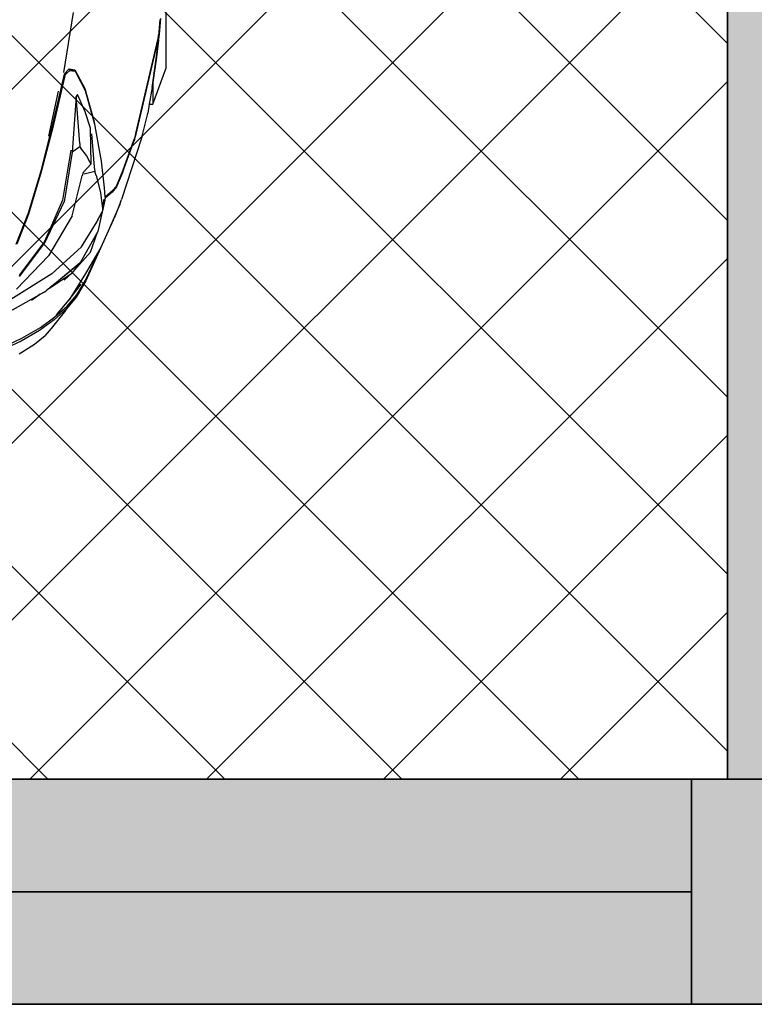
# Model space of a CAD drawing. Units: inches. Extents: x 2167 to 2589, y 1680 to 2489.
# Tile 14 of 38: x 2389 to 2419, y 1688 to 1727. Entities that reach past the tile are written whole.
import ezdxf

# ---------------------------------------------------------------- set-up
doc = ezdxf.new("R2010")
doc.units = ezdxf.units.IN
doc.header["$MEASUREMENT"] = 0
doc.layers.get('0').update_dxf_attribs({"color": 250})
doc.layers.add('A-FLOR-PATT', color=254, linetype='Continuous', lineweight=13, true_color=0xfeeab9)
for name, color, linetype, lineweight in [('A-WALL-PATT', 250, 'Continuous', 13), ('C-PRKG-VEHS', 8, 'Continuous', 13), ('C-PROP', 7, 'Continuous', 35), ('L-PVMT-PATT', 252, 'Continuous', 13), ('walls', 7, 'Continuous', 35)]:
    doc.layers.add(name, color=color, linetype=linetype, lineweight=lineweight)
doc.layers.add('Edges', color=250, linetype='Continuous')

# ---------------------------------------------------------------- blocks, each defined once
blk = doc.blocks.new('Nissan Qashqai pl')
at = {"layer": 'Edges'}
for p, q in [((10.9577, 12.8101), (11.1283, 12.8101)), ((11.1783, 12.7921), (11.1283, 12.8101)), ((11.0576, 12.8026), (11.0798, 12.8008)), ((11.0768, 12.8008), (11.059, 12.8023)), ((11.0811, 12.8004), (11.0768, 12.8008)), ((11.0798, 12.8008), (11.0872, 12.7999)), ((11.0827, 12.8001), (11.0811, 12.8004)), ((11.0827, 12.8001), (11.0813, 12.7998)), ((11.0836, 12.8002), (11.0827, 12.8001)), ((11.0856, 12.7994), (11.0827, 12.8001)), ((11.0872, 12.7999), (11.0836, 12.8002)), ((11.0836, 12.8002), (11.0882, 12.7992)), ((11.2196, 12.7681), (11.0856, 12.7994)), ((11.0883, 12.7998), (11.0872, 12.7999)), ((11.0882, 12.7992), (11.2222, 12.7676)), ((11.0883, 12.7998), (11.1123, 12.797)), ((11.1147, 12.7965), (11.0883, 12.7998)), ((11.1123, 12.797), (11.1475, 12.7921)), ((11.1547, 12.791), (11.1147, 12.7965)), ((11.1475, 12.7921), (11.1525, 12.7914)), ((11.1475, 12.7921), (11.1783, 12.7921)), ((11.1525, 12.7914), (11.1547, 12.791)), ((11.1547, 12.791), (11.1783, 12.787)), ((11.1783, 12.787), (11.1783, 12.7921)), ((11.1783, 12.787), (11.1906, 12.7849)), ((11.1906, 12.7849), (11.1909, 12.7849)), ((11.193, 12.7845), (11.1909, 12.7849)), ((11.2215, 12.7775), (11.193, 12.7845)), ((11.2247, 12.767), (11.2163, 12.7689)), ((11.22, 12.768), (11.2196, 12.7681)), ((11.2247, 12.767), (11.22, 12.768)), ((11.2247, 12.7764), (11.2215, 12.7775)), ((11.2222, 12.7676), (11.2271, 12.7664)), ((11.2247, 12.7764), (11.3124, 12.7479)), ((11.2253, 12.7668), (11.2247, 12.767)), ((11.2304, 12.7649), (11.2253, 12.7668)), ((11.2253, 12.7668), (11.2271, 12.7664)), ((11.2271, 12.7664), (11.2296, 12.7658)), ((11.2271, 12.7664), (11.2277, 12.7662)), ((11.2277, 12.7662), (11.2296, 12.7658)), ((11.2732, 12.7496), (11.2277, 12.7662)), ((11.2704, 12.7504), (11.2304, 12.7649)), ((11.2702, 12.7507), (11.2704, 12.7504)), ((11.2704, 12.7506), (11.2707, 12.7503)), ((11.2707, 12.7503), (11.2704, 12.7504)), ((11.2719, 12.7498), (11.2707, 12.7503)), ((11.2934, 12.741), (11.2719, 12.7498)), ((11.2732, 12.7496), (11.2946, 12.7409)), ((11.3, 12.735), (11.2934, 12.741)), ((11.2946, 12.7409), (11.3018, 12.7346)), ((11.3161, 12.7467), (11.3124, 12.7479)), ((11.3161, 12.7467), (11.3376, 12.7381)), ((11.3192, 12.7454), (11.3566, 12.7294)), ((11.3081, 12.7253), (11.3, 12.735)), ((11.3018, 12.7346), (11.3103, 12.7249)), ((11.3086, 12.7247), (11.3081, 12.7253)), ((11.3081, 12.7253), (11.3087, 12.7247)), ((11.3103, 12.7249), (11.3103, 12.7249)), ((11.3405, 12.7369), (11.3376, 12.7381)), ((11.3405, 12.7369), (11.3566, 12.7294)), ((11.3566, 12.7294), (11.3796, 12.7187)), ((11.2091, 12.7103), (11.2583, 12.7196)), ((11.2583, 12.7196), (11.2956, 12.7234)), ((11.2787, 12.7123), (11.2729, 12.7104)), ((11.2787, 12.7123), (11.3022, 12.7186)), ((11.2956, 12.7234), (11.3085, 12.7247)), ((11.3022, 12.7186), (11.3252, 12.7213)), ((11.3085, 12.7247), (11.3086, 12.7247)), ((11.3086, 12.7247), (11.3087, 12.7247)), ((11.3087, 12.7247), (11.3103, 12.7249)), ((11.3103, 12.7249), (11.3106, 12.7249)), ((11.3106, 12.7249), (11.314, 12.7238)), ((11.317, 12.7227), (11.3119, 12.7236)), ((11.3132, 12.7243), (11.3256, 12.7215)), ((11.314, 12.7238), (11.317, 12.7227)), ((11.314, 12.7238), (11.3242, 12.7216)), ((11.3242, 12.7216), (11.317, 12.7227)), ((11.3198, 12.7211), (11.3252, 12.7213)), ((11.3242, 12.7216), (11.3256, 12.7215)), ((11.3252, 12.7213), (11.3283, 12.7214)), ((11.3256, 12.7215), (11.3283, 12.7214)), ((11.3283, 12.7214), (11.3297, 12.7206)), ((11.3297, 12.7206), (11.3446, 12.7173)), ((11.3297, 12.7206), (11.3302, 12.7203)), ((11.3302, 12.7203), (11.3446, 12.7173)), ((11.3302, 12.7203), (11.3394, 12.7152)), ((11.3394, 12.7152), (11.3434, 12.7138)), ((11.3394, 12.7152), (11.342, 12.7137)), ((11.379, 12.6915), (11.3434, 12.7138)), ((11.3446, 12.7173), (11.3571, 12.7146)), ((11.3583, 12.7142), (11.3571, 12.7146)), ((11.3571, 12.7146), (11.3821, 12.7008)), ((11.3583, 12.7142), (11.3821, 12.7008)), ((11.3864, 12.7044), (11.3583, 12.7142)), ((11.3796, 12.7187), (11.4164, 12.6974)), ((11.3796, 12.7187), (11.3807, 12.7182)), ((11.3807, 12.7182), (11.4267, 12.6979)), ((11.4228, 12.6989), (11.3807, 12.7182)), ((11.156, 12.6966), (11.203, 12.7093)), ((11.1589, 12.6971), (11.2062, 12.7098)), ((11.2121, 12.7043), (11.189, 12.6968)), ((11.203, 12.7093), (11.2091, 12.7103)), ((11.2062, 12.7098), (11.2091, 12.7103)), ((11.2622, 12.7051), (11.2121, 12.7043)), ((11.2199, 12.706), (11.2666, 12.7097)), ((11.2505, 12.6987), (11.2401, 12.6908)), ((11.2601, 12.7037), (11.2505, 12.6987)), ((11.2622, 12.7051), (11.2601, 12.7037)), ((11.2743, 12.6942), (11.2622, 12.7051)), ((11.2666, 12.7097), (11.2729, 12.7104)), ((11.2729, 12.7104), (11.2766, 12.6957)), ((11.3821, 12.7008), (11.4014, 12.69)), ((11.4163, 12.6775), (11.3864, 12.7044)), ((11.4164, 12.6974), (11.4531, 12.6744)), ((11.4243, 12.6982), (11.4228, 12.6989)), ((11.4464, 12.6853), (11.4243, 12.6982)), ((11.4267, 12.6979), (11.4498, 12.6844)), ((11.1298, 12.6823), (11.156, 12.6966)), ((11.1319, 12.6827), (11.1365, 12.6851)), ((11.1365, 12.6851), (11.1589, 12.6971)), ((11.189, 12.6968), (11.1644, 12.6862)), ((11.1644, 12.6862), (11.1672, 12.6844)), ((11.2337, 12.6892), (11.1672, 12.6844)), ((11.1672, 12.6844), (11.2459, 12.6785)), ((11.2337, 12.6892), (11.2382, 12.6892)), ((11.2382, 12.6892), (11.2401, 12.6908)), ((11.2382, 12.6892), (11.2459, 12.6785)), ((11.2743, 12.6942), (11.2791, 12.6927)), ((11.335, 12.6786), (11.2791, 12.6927)), ((11.379, 12.6915), (11.417, 12.6499)), ((11.4014, 12.69), (11.4022, 12.6894)), ((11.4014, 12.69), (11.4265, 12.6594)), ((11.4022, 12.6894), (11.4163, 12.6775)), ((11.4022, 12.6894), (11.4265, 12.6594)), ((11.4531, 12.6744), (11.4314, 12.6911)), ((11.4624, 12.6717), (11.4464, 12.6853)), ((11.4498, 12.6844), (11.4662, 12.6706)), ((11.4681, 12.6691), (11.4498, 12.6844)), ((11.1336, 12.667), (11.0492, 12.6807)), ((11.1285, 12.6745), (11.1298, 12.6823)), ((11.1293, 12.6736), (11.1285, 12.6745)), ((11.1306, 12.6812), (11.1293, 12.6736)), ((11.1353, 12.6677), (11.1293, 12.6736)), ((11.1306, 12.6752), (11.1319, 12.6827)), ((11.1319, 12.6827), (11.1306, 12.6812)), ((11.1347, 12.671), (11.1306, 12.6752)), ((11.1366, 12.6691), (11.1347, 12.671)), ((11.2428, 12.6769), (11.3132, 12.6652)), ((11.2459, 12.6785), (11.3153, 12.6672)), ((11.335, 12.6786), (11.3915, 12.6453)), ((11.4366, 12.6471), (11.4163, 12.6775)), ((11.4163, 12.6775), (11.4259, 12.6674)), ((11.4742, 12.6567), (11.4531, 12.6744)), ((11.4774, 12.6543), (11.4624, 12.6717)), ((11.4662, 12.6706), (11.4815, 12.6531)), ((11.1358, 12.6676), (11.1353, 12.6677)), ((11.1358, 12.6676), (11.1366, 12.6691)), ((11.148, 12.665), (11.1358, 12.6676)), ((11.1401, 12.6682), (11.1366, 12.6691)), ((11.2066, 12.6527), (11.1401, 12.6682)), ((11.2063, 12.6515), (11.148, 12.665)), ((11.2232, 12.6458), (11.1598, 12.6594)), ((11.3132, 12.6652), (11.3715, 12.6398)), ((11.3733, 12.6404), (11.3153, 12.6672)), ((11.4265, 12.6594), (11.4366, 12.6471)), ((11.4681, 12.6691), (11.4936, 12.6491)), ((11.272, 12.6349), (11.2063, 12.6515)), ((11.2728, 12.6357), (11.2066, 12.6527)), ((11.3915, 12.6453), (11.4381, 12.6002)), ((11.417, 12.6499), (11.4529, 12.5922)), ((11.4366, 12.6471), (11.4408, 12.6419)), ((11.4408, 12.6419), (11.4411, 12.6414)), ((11.4924, 12.6339), (11.4774, 12.6543)), ((11.4815, 12.6531), (11.4963, 12.6328)), ((11.4936, 12.6491), (11.5033, 12.6408)), ((11.3311, 12.6172), (11.272, 12.6349)), ((11.3323, 12.6178), (11.2728, 12.6357)), ((11.3715, 12.6398), (11.4177, 12.6052)), ((11.4203, 12.6044), (11.3733, 12.6404)), ((11.4411, 12.6414), (11.4411, 12.6414)), ((11.4414, 12.6409), (11.4411, 12.6414)), ((11.4414, 12.6409), (11.447, 12.6315)), ((11.4455, 12.6336), (11.4414, 12.6409)), ((11.447, 12.6315), (11.4455, 12.6336)), ((11.4455, 12.6336), (11.4462, 12.6324)), ((11.447, 12.6315), (11.4462, 12.6324)), ((11.4732, 12.585), (11.4462, 12.6324)), ((11.447, 12.6315), (11.447, 12.6314)), ((11.4536, 12.6215), (11.447, 12.6314)), ((11.5074, 12.608), (11.4924, 12.6339)), ((11.4964, 12.6326), (11.4963, 12.6328)), ((11.4964, 12.6326), (11.5113, 12.6069)), ((11.5158, 12.6256), (11.5033, 12.6408)), ((11.3751, 12.5999), (11.3311, 12.6172)), ((11.3747, 12.6011), (11.3323, 12.6178)), ((11.5295, 12.6041), (11.5158, 12.6256)), ((11.4177, 12.6052), (11.4193, 12.6042)), ((11.5165, 12.5882), (11.5074, 12.608)), ((11.5113, 12.6068), (11.5113, 12.6069)), ((11.5113, 12.6068), (11.5206, 12.5869))]:
    blk.add_line(p, q, dxfattribs=at)
blk = doc.blocks.new('car')
blk.add_blockref('Nissan Qashqai pl', (-9.7433, -11.9151))
blk = doc.blocks.new('carr')
blk.add_blockref('car', (0.5124, -0.007))

msp = doc.modelspace()

# ---------------------------------------------------------------- hatches: boundary and pattern name
at = {"layer": 'A-FLOR-PATT'}
h = msp.add_hatch(color=256, dxfattribs=at)
h.dxf.hatch_style = 1
h.paths.add_polyline_path([(2525.548, 1864.695), (2455.041, 1864.695), (2455.041, 1855.153), (2455.041, 1830.653), (2525.548, 1830.653)])
h.paths.add_polyline_path([(2455.041, 1855.153), (2452.048, 1855.153), (2452.048, 1864.695), (2426.208, 1864.695), (2422.048, 1864.695), (2422.048, 1788.195), (2467.347, 1788.195), (2467.347, 1812.195), (2452.048, 1812.195), (2452.048, 1830.653), (2455.041, 1830.653)])
h.paths.add_polyline_path([(2419.685, 1779.195), (2417.548, 1779.195), (2417.548, 1696.695), (2419.685, 1696.695)])
at = {"layer": 'A-WALL-PATT'}
h = msp.add_hatch(color=256, dxfattribs=at)
h.dxf.hatch_style = 1
h.paths.add_polyline_path([(2575.048, 2029.695), (2422.048, 2029.695), (2422.048, 2161.695), (2427.018, 2161.695), (2427.018, 2161.941), (2427.018, 2166.195), (2417.548, 2166.195), (2417.548, 2025.195), (2575.048, 2025.195)])
h.paths.add_polyline_path([(2575.048, 2166.195), (2503.006, 2166.195), (2503.006, 2161.695), (2575.048, 2161.695)], flags=17)
h.paths.add_polyline_path([(2575.048, 2161.695), (2566.048, 2161.695), (2566.048, 2029.695), (2575.048, 2029.695)], flags=17)
h.paths.add_polyline_path([(2575.048, 2025.195), (2566.048, 2025.195), (2566.048, 1869.195), (2575.048, 1869.195)])
h.paths.add_polyline_path([(2575.048, 1869.195), (2566.048, 1869.195), (2447.7, 1869.195, -0.014764), (2447.737, 1867.924), (2447.737, 1864.695), (2575.048, 1864.695)])
h.paths.add_polyline_path([(2530.048, 1864.695), (2525.548, 1864.695), (2525.548, 1816.695), (2452.048, 1816.695), (2452.048, 1812.195), (2530.048, 1812.195)])
h.paths.add_polyline_path([(2455.041, 1830.653), (2452.048, 1830.653), (2452.048, 1816.695), (2455.041, 1816.695)], flags=17)
h.paths.add_polyline_path([(2575.048, 1864.695), (2566.048, 1864.695), (2566.048, 1788.195), (2456.097, 1788.195), (2456.097, 1783.941, -0.042065), (2455.697, 1779.195), (2527.685, 1779.195), (2527.685, 1687.695), (2532.185, 1687.695), (2532.185, 1779.195), (2575.048, 1779.195)])
h.paths.add_polyline_path([(2421.872, 1696.695), (2416.107, 1696.695), (2416.107, 1687.695), (2421.872, 1687.695)])
h.paths.add_polyline_path([(2375.607, 1696.695), (2369.843, 1696.695), (2369.843, 1687.695), (2375.607, 1687.695)])
h.paths.add_polyline_path([(2425.048, 2245.695), (2420.548, 2245.695), (2420.548, 2226.195), (2432.286, 2226.195), (2432.286, 2229.424), (2432.286, 2230.695), (2425.048, 2230.695)])
h.paths.add_polyline_path([(2224.048, 2151.195), (2318.548, 2151.195), (2318.548, 2177.304), (2314.783, 2177.304, -0.007324), (2314.048, 2177.315), (2314.048, 2155.695), (2224.048, 2155.695), (2224.048, 2157.455), (2215.048, 2157.455), (2215.048, 2103.585), (2218.974, 2103.585), (2224.048, 2103.585)])
at = {"layer": 'L-PVMT-PATT'}
h = msp.add_hatch(dxfattribs=at)
h.set_pattern_fill('ANSI37', color=256, scale=40)
h.paths.add_polyline_path([(2417.548, 1783.695), (2417.548, 1846.042), (2239.361, 1846.042), (2239.361, 1687.695), (2369.843, 1687.695), (2369.843, 1696.695), (2375.607, 1696.695), (2416.107, 1696.695), (2417.548, 1696.695)])
h = msp.add_hatch(color=256, dxfattribs=at)
h.dxf.hatch_style = 1
h.paths.add_polyline_path([(2416.107, 1696.695), (2375.607, 1696.695), (2375.607, 1692.195), (2416.107, 1692.195)])
h.paths.add_polyline_path([(2416.107, 1692.195), (2375.607, 1692.195), (2375.607, 1687.695), (2416.107, 1687.695)])

# ---------------------------------------------------------------- linework, layer by layer
at = {"layer": 'C-PROP'}
msp.add_line((2575.048, 1687.695), (2215.048, 1687.695), dxfattribs=at)
at = {"layer": 'walls'}
for p, q in [((2417.548, 1783.695), (2417.548, 1696.695)), ((2416.107, 1696.695), (2375.607, 1696.695)), ((2421.872, 1696.695), (2416.107, 1696.695)), ((2416.107, 1696.695), (2416.107, 1687.695)), ((2375.607, 1692.195), (2416.107, 1692.195))]:
    msp.add_line(p, q, dxfattribs=at)

# ---------------------------------------------------------------- block references
at = {"layer": 'C-PRKG-VEHS', "xscale": 28.42784210623918, "yscale": 28.42784210623918, "zscale": 28.42784210623918, "rotation": 270}
msp.add_blockref('carr', (2369.852, 1779.037), dxfattribs=at)

doc.saveas('drawing.dxf')
